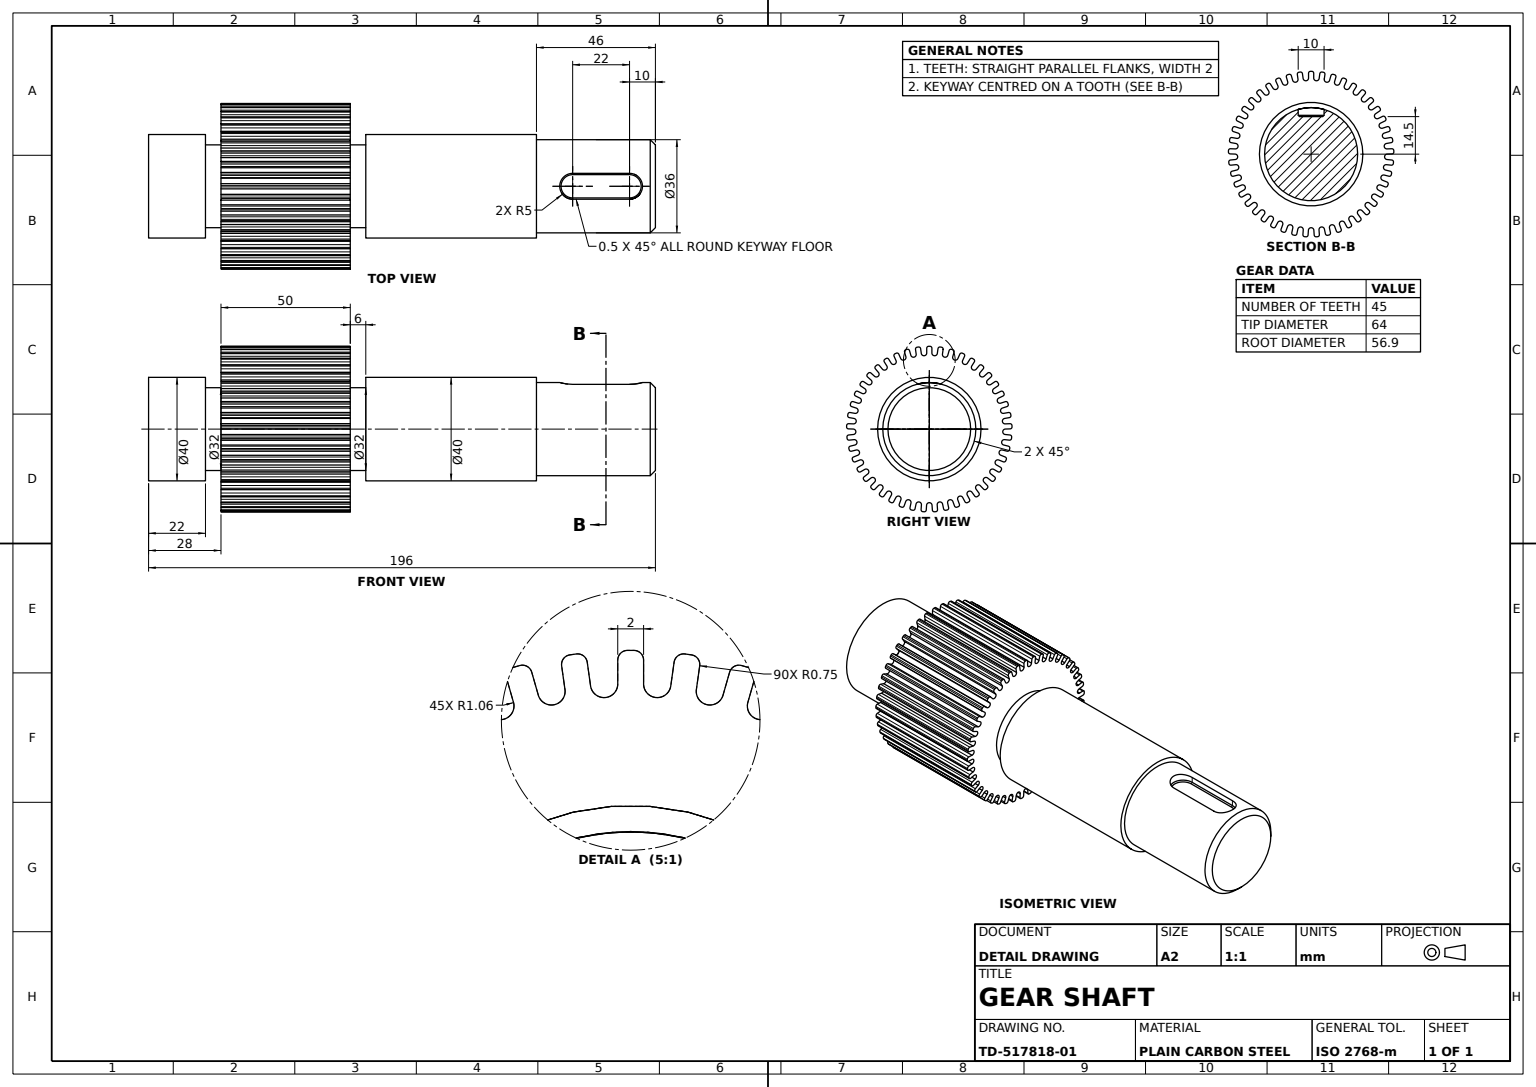
SolidWorks part; units mm, degrees
material "Plain Carbon Steel"
ref_plane "Front Plane" through (0, 0, 0) normal (0, 0, 1) x (1, 0, 0)
ref_plane "Top Plane" through (0, 0, 0) normal (0, 1, 0) x (1, 0, 0)
ref_plane "Right Plane" through (0, 0, 0) normal (1, 0, 0) x (0, 0, -1)
sketch "Shaft Profile Sketch" plane through (0, 0, 0) normal (0, 0, 1) x (1, 0, 0)
  line L0 (0, 0) -> (0, 20)
  line L1 (0, 20) -> (22, 20)
  line L2 (22, 20) -> (22, 16)
  line L3 (22, 16) -> (28, 16)
  line L4 (28, 16) -> (28, 32)
  line L5 (28, 32) -> (78, 32)
  line L6 (78, 32) -> (78, 16)
  line L7 (78, 16) -> (84, 16)
  line L8 (84, 16) -> (84, 20)
  line L9 (84, 20) -> (150, 20)
  line L10 (150, 20) -> (150, 18)
  line L11 (150, 18) -> (196, 18)
  line L12 (196, 18) -> (196, 0)
  line L13 (196, 0) -> (0, 0)
  dimension "D1" = 196
  dimension "D2" = 22
  dimension "D3" = 20
  dimension "D4" = 16
  dimension "D5" = 20
  dimension "D6" = 18
  dimension "D7" = 46
  dimension "D8" = 112
  dimension "D9" = 118
  dimension "D10" = 50
  dimension "D11" = 32
revolve "Shaft Body Revolve" add sketch "Shaft Profile Sketch" angle 360 about L13
sketch "Gear Teeth Sketch" plane through (78, 0, 0) normal (1, 0, 0) x (0, 0, -1)
  line L0 (-1, 29.4827) -> (-1, 31.249)
  line L1 (1, 29.4827) -> (1, 31.249)
  line L2 (3.1129, 29.335) -> (3.3588, 31.0841)
  line L3 (5.0935, 29.0566) -> (5.3393, 30.8057)
  line L4 (0, 35.1672) -> (0, -35.1672) construction
  line L5 (7.1653, 28.6162) -> (7.6521, 30.3141)
  line L6 (9.0878, 28.065) -> (9.5747, 29.7628)
  line L7 (11.0782, 27.3405) -> (11.7966, 28.9541)
  line L8 (12.9052, 26.5271) -> (13.6237, 28.1406)
  line L9 (14.7754, 25.5327) -> (15.7114, 27.0306)
  line L10 (16.4715, 24.4728) -> (17.4075, 25.9707)
  line L11 (18.1851, 23.2278) -> (19.3204, 24.5809)
  line L12 (19.7172, 21.9423) -> (20.8525, 23.2953)
  line L13 (21.2408, 20.4709) -> (22.5534, 21.6528)
  line L14 (22.579, 18.9846) -> (23.8917, 20.1665)
  line L15 (23.8831, 17.3156) -> (25.3474, 18.3033)
  line L16 (25.0015, 15.6575) -> (26.4658, 16.6452)
  line L17 (26.0605, 13.8232) -> (27.648, 14.5975)
  line L18 (26.9373, 12.0256) -> (28.5248, 12.7999)
  line L19 (27.7307, 10.0617) -> (29.4105, 10.6075)
  line L20 (28.3487, 8.1596) -> (30.0286, 8.7054)
  line L21 (28.8611, 6.1044) -> (30.6006, 6.4111)
  line L22 (29.2084, 4.1348) -> (30.9479, 4.4415)
  line L23 (29.4298, 2.0283) -> (31.1951, 2.09)
  line L24 (29.4996, 0.0295) -> (31.2649, 0.0912)
  line L25 (29.4257, -2.0873) -> (31.1823, -2.2719)
  line L26 (29.2167, -4.0763) -> (30.9733, -4.2609)
  line L27 (28.8489, -6.1622) -> (30.5627, -6.5895)
  line L28 (28.365, -8.1028) -> (30.0788, -8.5301)
  line L29 (27.7105, -10.1172) -> (29.3482, -10.7789)
  line L30 (26.9613, -11.9716) -> (28.599, -12.6333)
  line L31 (26.0328, -13.8753) -> (27.5624, -14.7585)
  line L32 (25.0328, -15.6074) -> (26.5624, -16.4905)
  line L33 (23.8483, -17.3634) -> (25.2402, -18.4508)
  line L34 (22.617, -18.9394) -> (24.0089, -20.0268)
  line L35 (21.1997, -20.5134) -> (22.4267, -21.784)
  line L36 (19.7611, -21.9027) -> (20.988, -23.1733)
  line L37 (18.1385, -23.2642) -> (19.1767, -24.6932)
  line L38 (16.5205, -24.4398) -> (17.5587, -25.8688)
  line L39 (14.7242, -25.5622) -> (15.5535, -27.1218)
  line L40 (12.9583, -26.5012) -> (13.7876, -28.0607)
  line L41 (11.0234, -27.3627) -> (11.6275, -29.0224)
  line L42 (9.144, -28.0467) -> (9.7481, -29.7065)
  line L43 (7.1079, -28.6305) -> (7.4752, -30.3582)
  line L44 (5.1517, -29.0463) -> (5.5189, -30.774)
  line L45 (3.0542, -29.3411) -> (3.1774, -31.1031)
  line L46 (1.059, -29.4806) -> (1.1823, -31.2426)
  line L47 (-1.059, -29.4806) -> (-1.1823, -31.2426)
  line L48 (-3.0542, -29.3411) -> (-3.1774, -31.1031)
  line L49 (-5.1517, -29.0463) -> (-5.5189, -30.774)
  line L50 (-7.1079, -28.6305) -> (-7.4752, -30.3582)
  line L51 (-9.144, -28.0467) -> (-9.7481, -29.7065)
  line L52 (-11.0234, -27.3627) -> (-11.6275, -29.0224)
  line L53 (-12.9583, -26.5012) -> (-13.7876, -28.0607)
  line L54 (-14.7242, -25.5622) -> (-15.5535, -27.1218)
  line L55 (-16.5205, -24.4398) -> (-17.5587, -25.8688)
  line L56 (-18.1385, -23.2642) -> (-19.1767, -24.6932)
  line L57 (-19.7611, -21.9027) -> (-20.988, -23.1733)
  line L58 (-21.1997, -20.5134) -> (-22.4267, -21.784)
  line L59 (-22.617, -18.9394) -> (-24.0089, -20.0268)
  line L60 (-23.8483, -17.3634) -> (-25.2402, -18.4508)
  line L61 (-25.0328, -15.6074) -> (-26.5624, -16.4905)
  line L62 (-26.0328, -13.8753) -> (-27.5624, -14.7585)
  line L63 (-26.9613, -11.9716) -> (-28.599, -12.6333)
  line L64 (-27.7105, -10.1172) -> (-29.3482, -10.7789)
  line L65 (-28.365, -8.1028) -> (-30.0788, -8.5301)
  line L66 (-28.8489, -6.1622) -> (-30.5627, -6.5895)
  line L67 (-29.2167, -4.0763) -> (-30.9733, -4.2609)
  line L68 (-29.4257, -2.0873) -> (-31.1823, -2.2719)
  line L69 (-29.4996, 0.0295) -> (-31.2649, 0.0912)
  line L70 (-29.4298, 2.0283) -> (-31.1951, 2.09)
  line L71 (-29.2084, 4.1348) -> (-30.9479, 4.4415)
  line L72 (-28.8611, 6.1044) -> (-30.6006, 6.4111)
  line L73 (-28.3487, 8.1596) -> (-30.0286, 8.7054)
  line L74 (-27.7307, 10.0617) -> (-29.4105, 10.6075)
  line L75 (-26.9373, 12.0256) -> (-28.5248, 12.7999)
  line L76 (-26.0605, 13.8232) -> (-27.648, 14.5975)
  line L77 (-25.0015, 15.6575) -> (-26.4658, 16.6452)
  line L78 (-23.8831, 17.3156) -> (-25.3474, 18.3033)
  line L79 (-22.579, 18.9846) -> (-23.8917, 20.1665)
  line L80 (-21.2408, 20.4709) -> (-22.5534, 21.6528)
  line L81 (-19.7172, 21.9423) -> (-20.8525, 23.2953)
  line L82 (-18.1851, 23.2278) -> (-19.3204, 24.5809)
  line L83 (-16.4715, 24.4728) -> (-17.4075, 25.9707)
  line L84 (-14.7754, 25.5327) -> (-15.7114, 27.0306)
  line L85 (-12.9052, 26.5271) -> (-13.6237, 28.1406)
  line L86 (-11.0782, 27.3405) -> (-11.7966, 28.9541)
  line L87 (-9.0878, 28.065) -> (-9.5747, 29.7628)
  line L88 (-7.1653, 28.6162) -> (-7.6521, 30.3141)
  line L89 (-5.0935, 29.0566) -> (-5.3393, 30.8057)
  line L90 (-3.1129, 29.335) -> (-3.3588, 31.0841)
  circle A1 centre (0, 0) radius 32 construction
  arc A2 (0.256, 31.999) -> (-0.256, 31.999) centre (0, 0) ccw
  arc A3 (-0.256, 31.999) -> (-1, 31.249) centre (-0.25, 31.249) ccw
  arc A4 (0.256, 31.999) -> (1, 31.249) centre (0.25, 31.249) cw
  arc A5 (4.1999, 31.7232) -> (3.3588, 31.0841) centre (4.1015, 30.9797) ccw
  arc A6 (4.7069, 31.6519) -> (5.3393, 30.8057) centre (4.5966, 30.9101) cw
  arc A7 (4.7069, 31.6519) -> (4.1999, 31.7232) centre (0, 0) ccw
  arc A8 (8.574, 30.83) -> (7.6521, 30.3141) centre (8.3731, 30.1074) ccw
  arc A9 (9.0662, 30.6888) -> (9.5747, 29.7628) centre (8.8537, 29.9696) cw
  arc A10 (9.0662, 30.6888) -> (8.574, 30.83) centre (0, 0) ccw
  arc A11 (12.7813, 29.3366) -> (11.7966, 28.9541) centre (12.4817, 28.6491) ccw
  arc A12 (13.249, 29.1284) -> (13.6237, 28.1406) centre (12.9385, 28.4457) cw
  arc A13 (13.249, 29.1284) -> (12.7813, 29.3366) centre (0, 0) ccw
  arc A14 (16.7398, 27.2723) -> (15.7114, 27.0306) centre (16.3474, 26.6331) ccw
  arc A15 (17.174, 27.001) -> (17.4075, 25.9707) centre (16.7715, 26.3682) cw
  arc A16 (17.174, 27.001) -> (16.7398, 27.2723) centre (0, 0) ccw
  arc A17 (20.3724, 24.6772) -> (19.3204, 24.5809) centre (19.895, 24.0988) ccw
  arc A18 (20.7647, 24.3481) -> (20.8525, 23.2953) centre (20.278, 23.7774) cw
  arc A19 (20.7647, 24.3481) -> (20.3724, 24.6772) centre (0, 0) ccw
  arc A20 (23.6086, 21.6017) -> (22.5534, 21.6528) centre (23.0552, 21.0954) ccw
  arc A21 (23.9512, 21.2212) -> (23.8917, 20.1665) centre (23.3898, 20.7239) cw
  arc A22 (23.9512, 21.2212) -> (23.6086, 21.6017) centre (0, 0) ccw
  arc A23 (26.3852, 18.1058) -> (25.3474, 18.3033) centre (25.7668, 17.6815) ccw
  arc A24 (26.6715, 17.6814) -> (26.4658, 16.6452) centre (26.0464, 17.267) cw
  arc A25 (26.6715, 17.6814) -> (26.3852, 18.1058) centre (0, 0) ccw
  arc A26 (28.6483, 14.2575) -> (27.648, 14.5975) centre (27.9768, 13.9234) ccw
  arc A27 (28.8727, 13.7973) -> (28.5248, 12.7999) centre (28.196, 13.474) cw
  arc A28 (28.8727, 13.7973) -> (28.6483, 14.2575) centre (0, 0) ccw
  arc A29 (30.3537, 10.1317) -> (29.4105, 10.6075) centre (29.6423, 9.8942) ccw
  arc A30 (30.5119, 9.6448) -> (30.0286, 8.7054) centre (29.7968, 9.4187) cw
  arc A31 (30.5119, 9.6448) -> (30.3537, 10.1317) centre (0, 0) ccw
  arc A32 (31.4684, 5.8087) -> (30.6006, 6.4111) centre (30.7308, 5.6725) ccw
  arc A33 (31.5573, 5.3045) -> (30.9479, 4.4415) centre (30.8177, 5.1801) cw
  arc A34 (31.5573, 5.3045) -> (31.4684, 5.8087) centre (0, 0) ccw
  arc A35 (31.9705, 1.3726) -> (31.1951, 2.09) centre (31.2212, 1.3404) ccw
  arc A36 (31.9884, 0.8609) -> (31.2649, 0.0912) centre (31.2387, 0.8407) cw
  arc A37 (31.9884, 0.8609) -> (31.9705, 1.3726) centre (0, 0) ccw
  arc A38 (31.8504, -3.0902) -> (31.1823, -2.2719) centre (31.1039, -3.0178) ccw
  arc A39 (31.7969, -3.5994) -> (30.9733, -4.2609) centre (31.0517, -3.515) cw
  arc A40 (31.7969, -3.5994) -> (31.8504, -3.0902) centre (0, 0) ccw
  arc A41 (31.1104, -7.4929) -> (30.5627, -6.5895) centre (30.3813, -7.3172) ccw
  arc A42 (30.9865, -7.9896) -> (30.0788, -8.5301) centre (30.2603, -7.8024) cw
  arc A43 (30.9865, -7.9896) -> (31.1104, -7.4929) centre (0, 0) ccw
  arc A44 (29.7648, -11.7497) -> (29.3482, -10.7789) centre (29.0672, -11.4743) ccw
  arc A45 (29.573, -12.2244) -> (28.599, -12.6333) centre (28.8799, -11.9379) cw
  arc A46 (29.573, -12.2244) -> (29.7648, -11.7497) centre (0, 0) ccw
  arc A47 (27.8399, -15.7778) -> (27.5624, -14.7585) centre (27.1874, -15.408) ccw
  arc A48 (27.5839, -16.2212) -> (26.5624, -16.4905) centre (26.9374, -15.841) cw
  arc A49 (27.5839, -16.2212) -> (27.8399, -15.7778) centre (0, 0) ccw
  arc A50 (25.3731, -19.4988) -> (25.2402, -18.4508) centre (24.7785, -19.0418) ccw
  arc A51 (25.0579, -19.9023) -> (24.0089, -20.0268) centre (24.4706, -19.4358) cw
  arc A52 (25.0579, -19.9023) -> (25.3731, -19.4988) centre (0, 0) ccw
  arc A53 (22.4125, -22.8403) -> (22.4267, -21.784) centre (21.8872, -22.305) ccw
  arc A54 (22.0442, -23.196) -> (20.988, -23.1733) centre (21.5275, -22.6523) cw
  arc A55 (22.0442, -23.196) -> (22.4125, -22.8403) centre (0, 0) ccw
  arc A56 (19.0156, -25.7372) -> (19.1767, -24.6932) centre (18.57, -25.134) ccw
  arc A57 (18.6014, -26.0382) -> (17.5587, -25.8688) centre (18.1654, -25.4279) cw
  arc A58 (18.6014, -26.0382) -> (19.0156, -25.7372) centre (0, 0) ccw
  arc A59 (15.2486, -28.1332) -> (15.5535, -27.1218) centre (14.8913, -27.4739) ccw
  arc A60 (14.7966, -28.3736) -> (13.7876, -28.0607) centre (14.4498, -27.7086) cw
  arc A61 (14.7966, -28.3736) -> (15.2486, -28.1332) centre (0, 0) ccw
  arc A62 (11.1849, -29.9816) -> (11.6275, -29.0224) centre (10.9227, -29.2789) ccw
  arc A63 (10.7037, -30.1568) -> (9.7481, -29.7065) centre (10.4529, -29.45) cw
  arc A64 (10.7037, -30.1568) -> (11.1849, -29.9816) centre (0, 0) ccw
  arc A65 (6.9034, -31.2465) -> (7.4752, -30.3582) centre (6.7416, -30.5142) ccw
  arc A66 (6.4026, -31.3529) -> (5.5189, -30.774) centre (6.2525, -30.6181) cw
  arc A67 (6.4026, -31.3529) -> (6.9034, -31.2465) centre (0, 0) ccw
  arc A68 (2.4875, -31.9032) -> (3.1774, -31.1031) centre (2.4292, -31.1554) ccw
  arc A69 (1.9768, -31.9389) -> (1.1823, -31.2426) centre (1.9304, -31.1903) cw
  arc A70 (1.9768, -31.9389) -> (2.4875, -31.9032) centre (0, 0) ccw
  arc A71 (-1.9768, -31.9389) -> (-1.1823, -31.2426) centre (-1.9304, -31.1903) ccw
  arc A72 (-2.4875, -31.9032) -> (-3.1774, -31.1031) centre (-2.4292, -31.1554) cw
  arc A73 (-2.4875, -31.9032) -> (-1.9768, -31.9389) centre (0, 0) ccw
  arc A74 (-6.4026, -31.3529) -> (-5.5189, -30.774) centre (-6.2525, -30.6181) ccw
  arc A75 (-6.9034, -31.2465) -> (-7.4752, -30.3582) centre (-6.7416, -30.5142) cw
  arc A76 (-6.9034, -31.2465) -> (-6.4026, -31.3529) centre (0, 0) ccw
  arc A77 (-10.7037, -30.1568) -> (-9.7481, -29.7065) centre (-10.4529, -29.45) ccw
  arc A78 (-11.1849, -29.9816) -> (-11.6275, -29.0224) centre (-10.9227, -29.2789) cw
  arc A79 (-11.1849, -29.9816) -> (-10.7037, -30.1568) centre (0, 0) ccw
  arc A80 (-14.7966, -28.3736) -> (-13.7876, -28.0607) centre (-14.4498, -27.7086) ccw
  arc A81 (-15.2486, -28.1332) -> (-15.5535, -27.1218) centre (-14.8913, -27.4739) cw
  arc A82 (-15.2486, -28.1332) -> (-14.7966, -28.3736) centre (0, 0) ccw
  arc A83 (-18.6014, -26.0382) -> (-17.5587, -25.8688) centre (-18.1654, -25.4279) ccw
  arc A84 (-19.0156, -25.7372) -> (-19.1767, -24.6932) centre (-18.57, -25.134) cw
  arc A85 (-19.0156, -25.7372) -> (-18.6014, -26.0382) centre (0, 0) ccw
  arc A86 (-22.0442, -23.196) -> (-20.988, -23.1733) centre (-21.5275, -22.6523) ccw
  arc A87 (-22.4125, -22.8403) -> (-22.4267, -21.784) centre (-21.8872, -22.305) cw
  arc A88 (-22.4125, -22.8403) -> (-22.0442, -23.196) centre (0, 0) ccw
  arc A89 (-25.0579, -19.9023) -> (-24.0089, -20.0268) centre (-24.4706, -19.4358) ccw
  arc A90 (-25.3731, -19.4988) -> (-25.2402, -18.4508) centre (-24.7785, -19.0418) cw
  arc A91 (-25.3731, -19.4988) -> (-25.0579, -19.9023) centre (0, 0) ccw
  arc A92 (-27.5839, -16.2212) -> (-26.5624, -16.4905) centre (-26.9374, -15.841) ccw
  arc A93 (-27.8399, -15.7778) -> (-27.5624, -14.7585) centre (-27.1874, -15.408) cw
  arc A94 (-27.8399, -15.7778) -> (-27.5839, -16.2212) centre (0, 0) ccw
  arc A95 (-29.573, -12.2244) -> (-28.599, -12.6333) centre (-28.8799, -11.9379) ccw
  arc A96 (-29.7648, -11.7497) -> (-29.3482, -10.7789) centre (-29.0672, -11.4743) cw
  arc A97 (-29.7648, -11.7497) -> (-29.573, -12.2244) centre (0, 0) ccw
  arc A98 (-30.9865, -7.9896) -> (-30.0788, -8.5301) centre (-30.2603, -7.8024) ccw
  arc A99 (-31.1104, -7.4929) -> (-30.5627, -6.5895) centre (-30.3813, -7.3172) cw
  arc A100 (-31.1104, -7.4929) -> (-30.9865, -7.9896) centre (0, 0) ccw
  arc A101 (-31.7969, -3.5994) -> (-30.9733, -4.2609) centre (-31.0517, -3.515) ccw
  arc A102 (-31.8504, -3.0902) -> (-31.1823, -2.2719) centre (-31.1039, -3.0178) cw
  arc A103 (-31.8504, -3.0902) -> (-31.7969, -3.5994) centre (0, 0) ccw
  arc A104 (-31.9884, 0.8609) -> (-31.2649, 0.0912) centre (-31.2387, 0.8407) ccw
  arc A105 (-31.9705, 1.3726) -> (-31.1951, 2.09) centre (-31.2212, 1.3404) cw
  arc A106 (-31.9705, 1.3726) -> (-31.9884, 0.8609) centre (0, 0) ccw
  arc A107 (-31.5573, 5.3045) -> (-30.9479, 4.4415) centre (-30.8177, 5.1801) ccw
  arc A108 (-31.4684, 5.8087) -> (-30.6006, 6.4111) centre (-30.7308, 5.6725) cw
  arc A109 (-31.4684, 5.8087) -> (-31.5573, 5.3045) centre (0, 0) ccw
  arc A110 (-30.5119, 9.6448) -> (-30.0286, 8.7054) centre (-29.7968, 9.4187) ccw
  arc A111 (-30.3537, 10.1317) -> (-29.4105, 10.6075) centre (-29.6423, 9.8942) cw
  arc A112 (-30.3537, 10.1317) -> (-30.5119, 9.6448) centre (0, 0) ccw
  arc A113 (-28.8727, 13.7973) -> (-28.5248, 12.7999) centre (-28.196, 13.474) ccw
  arc A114 (-28.6483, 14.2575) -> (-27.648, 14.5975) centre (-27.9768, 13.9234) cw
  arc A115 (-28.6483, 14.2575) -> (-28.8727, 13.7973) centre (0, 0) ccw
  arc A116 (-26.6715, 17.6814) -> (-26.4658, 16.6452) centre (-26.0464, 17.267) ccw
  arc A117 (-26.3852, 18.1058) -> (-25.3474, 18.3033) centre (-25.7668, 17.6815) cw
  arc A118 (-26.3852, 18.1058) -> (-26.6715, 17.6814) centre (0, 0) ccw
  arc A119 (-23.9512, 21.2212) -> (-23.8917, 20.1665) centre (-23.3898, 20.7239) ccw
  arc A120 (-23.6086, 21.6017) -> (-22.5534, 21.6528) centre (-23.0552, 21.0954) cw
  arc A121 (-23.6086, 21.6017) -> (-23.9512, 21.2212) centre (0, 0) ccw
  arc A122 (-20.7647, 24.3481) -> (-20.8525, 23.2953) centre (-20.278, 23.7774) ccw
  arc A123 (-20.3724, 24.6772) -> (-19.3204, 24.5809) centre (-19.895, 24.0988) cw
  arc A124 (-20.3724, 24.6772) -> (-20.7647, 24.3481) centre (0, 0) ccw
  arc A125 (-17.174, 27.001) -> (-17.4075, 25.9707) centre (-16.7715, 26.3682) ccw
  arc A126 (-16.7398, 27.2723) -> (-15.7114, 27.0306) centre (-16.3474, 26.6331) cw
  arc A127 (-16.7398, 27.2723) -> (-17.174, 27.001) centre (0, 0) ccw
  arc A128 (-13.249, 29.1284) -> (-13.6237, 28.1406) centre (-12.9385, 28.4457) ccw
  arc A129 (-12.7813, 29.3366) -> (-11.7966, 28.9541) centre (-12.4817, 28.6491) cw
  arc A130 (-12.7813, 29.3366) -> (-13.249, 29.1284) centre (0, 0) ccw
  arc A131 (-9.0662, 30.6888) -> (-9.5747, 29.7628) centre (-8.8537, 29.9696) ccw
  arc A132 (-8.574, 30.83) -> (-7.6521, 30.3141) centre (-8.3731, 30.1074) cw
  arc A133 (-8.574, 30.83) -> (-9.0662, 30.6888) centre (0, 0) ccw
  arc A134 (-4.7069, 31.6519) -> (-5.3393, 30.8057) centre (-4.5966, 30.9101) ccw
  arc A135 (-4.1999, 31.7232) -> (-3.3588, 31.0841) centre (-4.1015, 30.9797) cw
  arc A136 (-4.1999, 31.7232) -> (-4.7069, 31.6519) centre (0, 0) ccw
  arc A137 (-3.1129, 29.335) -> (-1, 29.4827) centre (-2.0565, 29.4088) ccw
  arc A138 (1, 29.4827) -> (3.1129, 29.335) centre (2.0565, 29.4088) ccw
  arc A139 (5.0935, 29.0566) -> (7.1653, 28.6162) centre (6.1294, 28.8364) ccw
  arc A140 (9.0878, 28.065) -> (11.0782, 27.3405) centre (10.083, 27.7027) ccw
  arc A141 (12.9052, 26.5271) -> (14.7754, 25.5327) centre (13.8403, 26.0299) ccw
  arc A142 (16.4715, 24.4728) -> (18.1851, 23.2278) centre (17.3283, 23.8503) ccw
  arc A143 (19.7172, 21.9423) -> (21.2408, 20.4709) centre (20.479, 21.2066) ccw
  arc A144 (22.579, 18.9846) -> (23.8831, 17.3156) centre (23.2311, 18.1501) ccw
  arc A145 (25.0015, 15.6575) -> (26.0605, 13.8232) centre (25.531, 14.7403) ccw
  arc A146 (26.9373, 12.0256) -> (27.7307, 10.0617) centre (27.334, 11.0436) ccw
  arc A147 (28.3487, 8.1596) -> (28.8611, 6.1044) centre (28.6049, 7.132) ccw
  arc A148 (29.2084, 4.1348) -> (29.4298, 2.0283) centre (29.3191, 3.0816) ccw
  arc A149 (29.4996, 0.0295) -> (29.4257, -2.0873) centre (29.4627, -1.0289) ccw
  arc A150 (29.2167, -4.0763) -> (28.8489, -6.1622) centre (29.0328, -5.1193) ccw
  arc A151 (28.365, -8.1028) -> (27.7105, -10.1172) centre (28.0378, -9.11) ccw
  arc A152 (26.9613, -11.9716) -> (26.0328, -13.8753) centre (26.497, -12.9235) ccw
  arc A153 (25.0328, -15.6074) -> (23.8483, -17.3634) centre (24.4406, -16.4854) ccw
  arc A154 (22.617, -18.9394) -> (21.1997, -20.5134) centre (21.9084, -19.7264) ccw
  arc A155 (19.7611, -21.9027) -> (18.1385, -23.2642) centre (18.9498, -22.5835) ccw
  arc A156 (16.5205, -24.4398) -> (14.7242, -25.5622) centre (15.6224, -25.001) ccw
  arc A157 (12.9583, -26.5012) -> (11.0234, -27.3627) centre (11.9909, -26.9319) ccw
  arc A158 (9.144, -28.0467) -> (7.1079, -28.6305) centre (8.126, -28.3386) ccw
  arc A159 (5.1517, -29.0463) -> (3.0542, -29.3411) centre (4.1029, -29.1937) ccw
  arc A160 (1.059, -29.4806) -> (-1.059, -29.4806) centre (0, -29.4806) ccw
  arc A161 (-3.0542, -29.3411) -> (-5.1517, -29.0463) centre (-4.1029, -29.1937) ccw
  arc A162 (-7.1079, -28.6305) -> (-9.144, -28.0467) centre (-8.126, -28.3386) ccw
  arc A163 (-11.0234, -27.3627) -> (-12.9583, -26.5012) centre (-11.9909, -26.9319) ccw
  arc A164 (-14.7242, -25.5622) -> (-16.5205, -24.4398) centre (-15.6224, -25.001) ccw
  arc A165 (-18.1385, -23.2642) -> (-19.7611, -21.9027) centre (-18.9498, -22.5835) ccw
  arc A166 (-21.1997, -20.5134) -> (-22.617, -18.9394) centre (-21.9084, -19.7264) ccw
  arc A167 (-23.8483, -17.3634) -> (-25.0328, -15.6074) centre (-24.4406, -16.4854) ccw
  arc A168 (-26.0328, -13.8753) -> (-26.9613, -11.9716) centre (-26.497, -12.9235) ccw
  arc A169 (-27.7105, -10.1172) -> (-28.365, -8.1028) centre (-28.0378, -9.11) ccw
  arc A170 (-28.8489, -6.1622) -> (-29.2167, -4.0763) centre (-29.0328, -5.1193) ccw
  arc A171 (-29.4257, -2.0873) -> (-29.4996, 0.0295) centre (-29.4627, -1.0289) ccw
  arc A172 (-29.4298, 2.0283) -> (-29.2084, 4.1348) centre (-29.3191, 3.0816) ccw
  arc A173 (-28.8611, 6.1044) -> (-28.3487, 8.1596) centre (-28.6049, 7.132) ccw
  arc A174 (-27.7307, 10.0617) -> (-26.9373, 12.0256) centre (-27.334, 11.0436) ccw
  arc A175 (-26.0605, 13.8232) -> (-25.0015, 15.6575) centre (-25.531, 14.7403) ccw
  arc A176 (-23.8831, 17.3156) -> (-22.579, 18.9846) centre (-23.2311, 18.1501) ccw
  arc A177 (-21.2408, 20.4709) -> (-19.7172, 21.9423) centre (-20.479, 21.2066) ccw
  arc A178 (-18.1851, 23.2278) -> (-16.4715, 24.4728) centre (-17.3283, 23.8503) ccw
  arc A179 (-14.7754, 25.5327) -> (-12.9052, 26.5271) centre (-13.8403, 26.0299) ccw
  arc A180 (-11.0782, 27.3405) -> (-9.0878, 28.065) centre (-10.083, 27.7027) ccw
  arc A181 (-7.1653, 28.6162) -> (-5.0935, 29.0566) centre (-6.1294, 28.8364) ccw
  point P366 (0, 0)
  point P500 (0, 0)
  dimension "D1" = 45
  dimension "D4" = 1.5
  dimension "D5" = 0.25
  dimension "D3" = 1.059
  dimension "D2" = 45
extrude "Gear Teeth Cut" cut sketch "Gear Teeth Sketch" against normal blind 50 flip side to cut
ref_plane "Keyway Plane" through (0, 14.5, 0) normal (0, 1, 0) x (1, 0, 0)
sketch "Keyway Sketch" plane through (0, 14.5, 0) normal (0, 1, 0) x (1, 0, 0)
  line L0 (164, 0) -> (186, 0) construction
  line L1 (164, 5) -> (186, 5)
  line L2 (164, -5) -> (186, -5)
  line L5 (196, -18) -> (196, 18) construction
  arc A0 (164, 5) -> (164, -5) centre (164, 0) ccw
  arc A1 (186, -5) -> (186, 5) centre (186, 0) ccw
  point P2 (175, 0)
  point P8 (191, 0)
  dimension "D2" = 5
  dimension "D3" = 5
  dimension "D1" = 22
extrude "Keyway Cut 5x22" cut sketch "Keyway Sketch" along normal blind 7
chamfer "Shaft Edge Chamfer 2mm" distance 2 angle 45 1 edges at (196, 0, -18)
chamfer "Keyway Edge Chamfer 0.5mm" distance 0.5 angle 45 4 edges at (175, 14.5, -5) (191, 14.5, 0) (175, 14.5, 5) (159, 14.5, 0)
